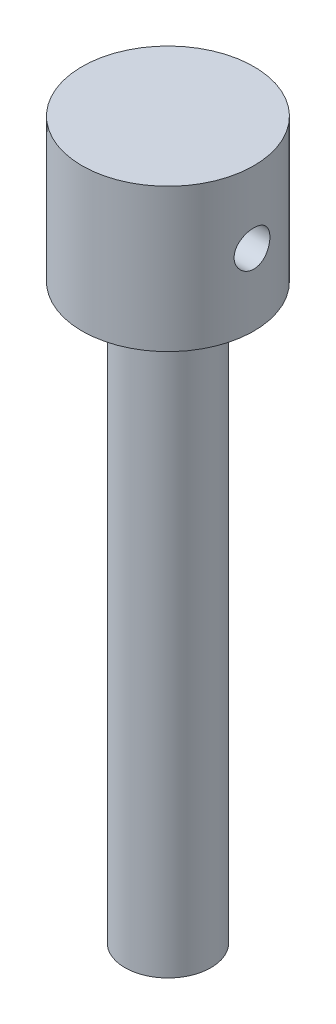
from build123d import *

# Parameters (mm, degrees)
SHAFT_PROFILE_R      = 6
SHAFT_L80_DEPTH      = 80
HEAD_PROFILE_R       = 12
HEAD_24_X_20_DEPTH   = 20
CROSS_HOLE_PROFILE_R = 2.5
CROSS_HOLE_DEPTH     = 25


with BuildPart() as part:
    # Shaft Profile → Shaft L80 (new body)
    with BuildSketch(Plane(origin=(0, 0, 0), x_dir=(1, 0, 0), z_dir=(0, 1, 0))):
        with Locations(Location((0, 0, 0), (0, 0, 270))):
            Circle(SHAFT_PROFILE_R)
    extrude(amount=SHAFT_L80_DEPTH)

    # Head Profile → Head Ø24 x 20 (add)
    with BuildSketch(Plane(origin=(0, 80, 0), x_dir=(1, 0, 0), z_dir=(0, 1, 0))):
        with Locations(Location((0, 0, 0), (0, 0, 270))):
            Circle(HEAD_PROFILE_R)
    extrude(amount=HEAD_24_X_20_DEPTH)

    # Cross Hole Profile → Cross Hole (cut, symmetric)
    with BuildSketch(Plane(origin=(0, 0, 0), x_dir=(0, 0, -1), z_dir=(1, 0, 0))):
        with Locations((0, 90)):
            Circle(CROSS_HOLE_PROFILE_R)
    extrude(amount=CROSS_HOLE_DEPTH, both=True, mode=Mode.SUBTRACT)


solid = part.part
